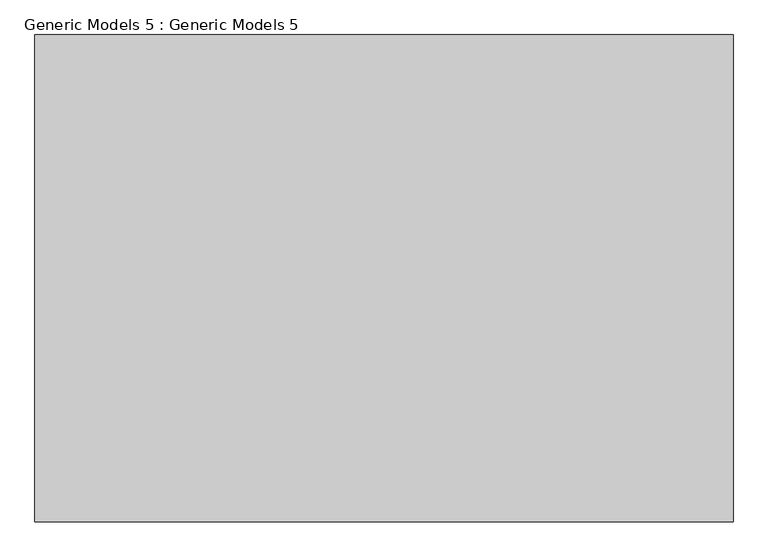
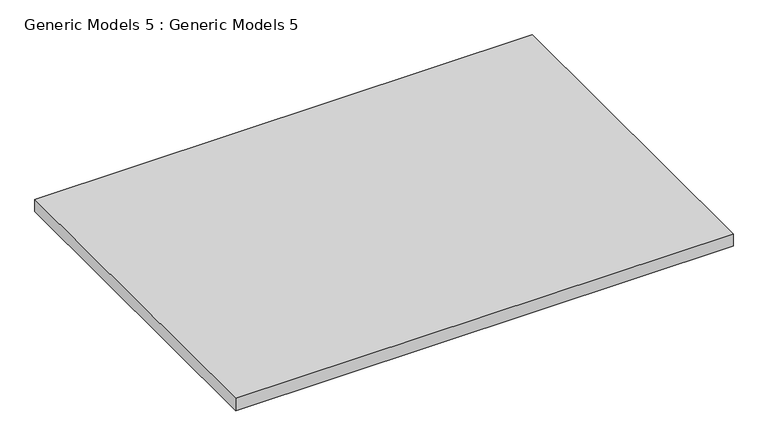
"""IFC4 building model written with IfcOpenShell, lengths in millimetres: proxy geometry, Generic Models 5 : Generic Models 5."""

from ifc_helpers import new_model, si_unit, frame, origin, place, context, project, spatial, polyline, outline, extrude, source, transform, mapped, element, save


def generic_models_5_generic_models_5_0426171c(model_context):
    return source(origin(), model_context, "Body", "SweptSolid", [
        extrude(outline(polyline([(7778.9999715, -6698.7302299), (-4006.6000285, -6698.7302299), (-4006.6000285, 1530.8697701), (7778.9999715, 1530.8697701), (7778.9999715, -6698.7302299)])), frame((0.0, 0.0, 63122.7531058), z_axis=(0.0, 0.0, 1.0), x_axis=(1.0, 0.0, 0.0)), (0.0, 0.0, 1.0), 304.8),
    ])


if __name__ == "__main__":
    model = new_model("IFC4")
    model_context = context("Model", 3, world=origin())
    ifc_project = project(units=[si_unit("LENGTHUNIT", "METRE", prefix="MILLI")], contexts=[model_context])
    site = spatial("IfcSite", under=ifc_project)
    building = spatial("IfcBuilding", under=site)
    placement = place(None, origin())
    generic_models_5_generic_models_5_shape = generic_models_5_generic_models_5_0426171c(model_context)
    element("IfcBuildingElementProxy", 1, Name="Generic Models 5 : Generic Models 5", ObjectType="Generic Models 5 : Generic Models 5", at=placement, inside=building, context=model_context, shape_type="MappedRepresentation", body=[
        mapped(generic_models_5_generic_models_5_shape, transform((0.0, 0.0, 0.0), x_axis=(1.0, 0.0, 0.0), y_axis=(0.0, 1.0, 0.0), z_axis=(0.0, 0.0, 1.0))),
    ])
    save(model, "model.ifc")
